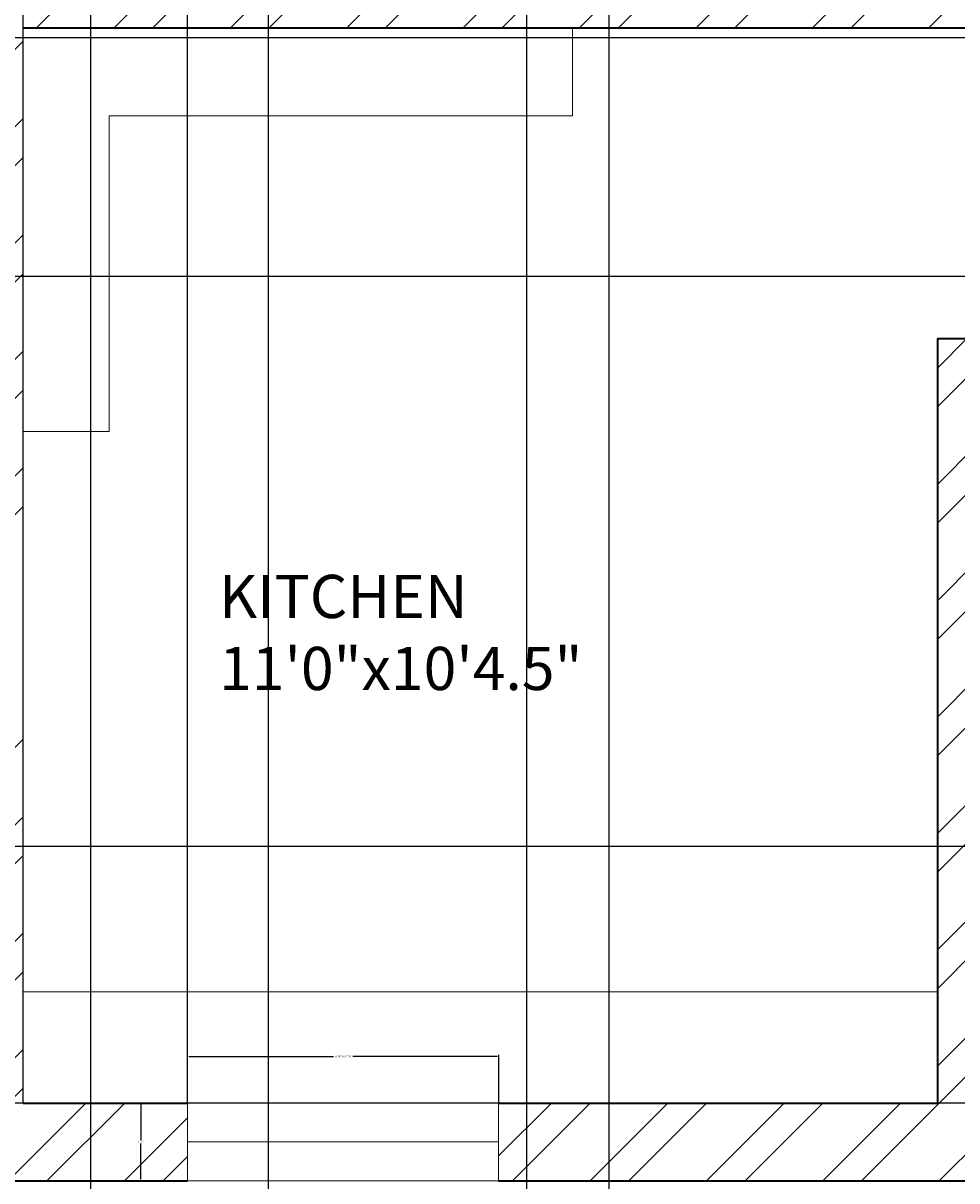
# Model space of a CAD drawing. Units: inches. Extents: x 1748 to 2382, y 1346 to 2284.
# Tile 3 of 26: x 1901 to 2009, y 1468 to 1602. Entities that reach past the tile are written whole.
import ezdxf

# ---------------------------------------------------------------- set-up
doc = ezdxf.new("R2010")
doc.units = ezdxf.units.IN
for name, color, linetype, lineweight in [('A-ANNO-DIMS', 2, 'Continuous', 18), ('A-AREA-IDEN', 7, 'Continuous', 18), ('A-FLOR-CASE', 32, 'Continuous', 18), ('A-GLAZ', 191, 'Continuous', 18), ('A-WALL', 7, 'Continuous', 35), ('A-WALL-PATT', 9, 'Continuous', 13)]:
    doc.layers.add(name, color=color, linetype=linetype, lineweight=lineweight)
doc.styles.get("Standard").update_dxf_attribs({"font": 'arial.ttf'})
doc.dimstyles.get("Standard").update_dxf_attribs({"dimtxt": 0.18, "dimasz": 0.18, "dimexe": 0.18, "dimexo": 0.0625, "dimgap": 0.09, "dimtad": 0, "dimtih": 1, "dimtoh": 1, "dimdec": 4, "dimzin": 0, "dimdsep": 46, "dimtxsty": 'Standard', "dimcen": 0.09, "dimadec": 0, "dimazin": 0, "dimtfac": 1, "dimtdec": 4, "dimtofl": 0, "dimtmove": 0, "dimatfit": 3, "dimfxl": 1, "dimtolj": 1, "dimtzin": 0, "dimarcsym": 0})

# ---------------------------------------------------------------- blocks, each defined once
blk = doc.blocks.new('WIN-36-DEEP')
for p, q in [((0, 9), (0, 0)), ((0, 9), (36, 9)), ((36, 4.5), (36, 9)), ((36, 9), (36, 0)), ((0, 0), (0, 4.5)), ((0, 4.5), (36, 4.5)), ((36, 0), (0, 0))]:
    blk.add_line(p, q)
blk = doc.blocks.new('*D28')
at = {"layer": 'A-ANNO-DIMS', "color": 0, "lineweight": -2, "transparency": 16777216}
for p, q in [((1919.68, 1476.91), (1919.68, 1482.43)), ((1955.68, 1476.91), (1955.68, 1482.43)), ((1919.86, 1482.25), (1936.56, 1482.25)), ((1955.5, 1482.25), (1938.8, 1482.25))]:
    blk.add_line(p, q, dxfattribs=at)
at = {"layer": 'A-ANNO-DIMS', "color": 0, "transparency": 16777216}
for points in [[(1919.86, 1482.28), (1919.86, 1482.22), (1919.68, 1482.25)], [(1955.5, 1482.28), (1955.5, 1482.22), (1955.68, 1482.25)]]:
    blk.add_solid(points, dxfattribs=at)
at = {"layer": 'Defpoints', "color": 0, "transparency": 16777216}
for p in [(1955.68, 1482.25), (1919.68, 1476.85), (1955.68, 1476.85)]:
    blk.add_point(p, dxfattribs=at)
at = {"layer": 'A-ANNO-DIMS', "color": 0, "transparency": 16777216, "insert": (1937.68, 1482.25), "char_height": 0.18, "attachment_point": 5}
blk.add_mtext('\\A1;WINDOW 36 TYP.', dxfattribs=at)
blk = doc.blocks.new('*D29')
at = {"layer": 'A-ANNO-DIMS', "color": 0, "lineweight": -2, "transparency": 16777216}
for p, q in [((1919.62, 1476.85), (1914.1, 1476.85)), ((1914.28, 1476.67), (1914.28, 1472.53)), ((1914.28, 1468.03), (1914.28, 1472.17)), ((1919.62, 1467.85), (1914.1, 1467.85))]:
    blk.add_line(p, q, dxfattribs=at)
at = {"layer": 'A-ANNO-DIMS', "color": 0, "transparency": 16777216}
for points in [[(1914.25, 1476.67), (1914.31, 1476.67), (1914.28, 1476.85)], [(1914.25, 1468.03), (1914.31, 1468.03), (1914.28, 1467.85)]]:
    blk.add_solid(points, dxfattribs=at)
at = {"layer": 'Defpoints', "color": 0, "transparency": 16777216}
for p in [(1914.28, 1476.85), (1919.68, 1476.85), (1919.68, 1467.85)]:
    blk.add_point(p, dxfattribs=at)
at = {"layer": 'A-ANNO-DIMS', "color": 0, "transparency": 16777216, "insert": (1914.28, 1472.35), "char_height": 0.18, "attachment_point": 5}
blk.add_mtext('\\A1;9 TYP.', dxfattribs=at)
blk = doc.blocks.new('*D50')
at = {"layer": 'A-ANNO-DIMS', "color": 0, "lineweight": -2, "transparency": 16777216}
for p, q in [((1869.96, 2223.79), (1869.96, 1360.47)), ((1908.44, 2223.79), (1908.44, 1360.47)), ((1870.14, 1360.65), (1888.81, 1360.65)), ((1908.26, 1360.65), (1889.6, 1360.65))]:
    blk.add_line(p, q, dxfattribs=at)
at = {"layer": 'A-ANNO-DIMS', "color": 0, "transparency": 16777216}
for points in [[(1870.14, 1360.68), (1870.14, 1360.62), (1869.96, 1360.65)], [(1908.26, 1360.68), (1908.26, 1360.62), (1908.44, 1360.65)]]:
    blk.add_solid(points, dxfattribs=at)
at = {"layer": 'Defpoints', "color": 0, "transparency": 16777216}
for p in [(1869.96, 2223.85), (1908.44, 2223.85), (1908.44, 1360.65)]:
    blk.add_point(p, dxfattribs=at)
at = {"layer": 'A-ANNO-DIMS', "color": 0, "transparency": 16777216, "insert": (1889.2, 1360.65), "char_height": 0.18, "attachment_point": 5}
blk.add_mtext('\\A1;38.48', dxfattribs=at)
blk = doc.blocks.new('*D51')
at = {"layer": 'A-ANNO-DIMS', "color": 0, "lineweight": -2, "transparency": 16777216}
for p, q in [((1968.44, 2223.79), (1968.44, 1360.47)), ((2040.07, 2223.79), (2040.07, 1360.47)), ((1968.62, 1360.65), (2003.86, 1360.65)), ((2039.89, 1360.65), (2004.65, 1360.65))]:
    blk.add_line(p, q, dxfattribs=at)
at = {"layer": 'A-ANNO-DIMS', "color": 0, "transparency": 16777216}
for points in [[(1968.62, 1360.68), (1968.62, 1360.62), (1968.44, 1360.65)], [(2039.89, 1360.68), (2039.89, 1360.62), (2040.07, 1360.65)]]:
    blk.add_solid(points, dxfattribs=at)
at = {"layer": 'Defpoints', "color": 0, "transparency": 16777216}
for p in [(1968.44, 2223.85), (2040.07, 2223.85), (2040.07, 1360.65)]:
    blk.add_point(p, dxfattribs=at)
at = {"layer": 'A-ANNO-DIMS', "color": 0, "transparency": 16777216, "insert": (2004.26, 1360.65), "char_height": 0.18, "attachment_point": 5}
blk.add_mtext('\\A1;71.62', dxfattribs=at)
blk = doc.blocks.new('*D54')
at = {"layer": 'A-ANNO-DIMS', "color": 0, "lineweight": -2, "transparency": 16777216}
for p, q in [((2288.4, 1506.57), (1779.88, 1506.57)), ((1780.06, 1506.39), (1780.06, 1491.89)), ((1780.06, 1477.03), (1780.06, 1491.53)), ((2288.4, 1476.85), (1779.88, 1476.85))]:
    blk.add_line(p, q, dxfattribs=at)
at = {"layer": 'A-ANNO-DIMS', "color": 0, "transparency": 16777216}
for points in [[(1780.03, 1506.39), (1780.09, 1506.39), (1780.06, 1506.57)], [(1780.03, 1477.03), (1780.09, 1477.03), (1780.06, 1476.85)]]:
    blk.add_solid(points, dxfattribs=at)
at = {"layer": 'Defpoints', "color": 0, "transparency": 16777216}
for p in [(1780.06, 1506.57), (2288.46, 1506.57), (2288.46, 1476.85)]:
    blk.add_point(p, dxfattribs=at)
at = {"layer": 'A-ANNO-DIMS', "color": 0, "transparency": 16777216, "insert": (1780.06, 1491.71), "char_height": 0.18, "attachment_point": 5}
blk.add_mtext('\\A1;29.716', dxfattribs=at)
blk = doc.blocks.new('*D64')
at = {"layer": 'A-ANNO-DIMS', "color": 0, "lineweight": -2, "transparency": 16777216}
for p, q in [((1900.64, 1476.91), (1900.64, 2274.93)), ((1900.82, 2274.75), (1909.7, 2274.75)), ((1919.5, 2274.75), (1910.62, 2274.75)), ((1919.68, 1476.91), (1919.68, 2274.93))]:
    blk.add_line(p, q, dxfattribs=at)
at = {"layer": 'A-ANNO-DIMS', "color": 0, "transparency": 16777216}
for points in [[(1900.82, 2274.78), (1900.82, 2274.72), (1900.64, 2274.75)], [(1919.5, 2274.78), (1919.5, 2274.72), (1919.68, 2274.75)]]:
    blk.add_solid(points, dxfattribs=at)
at = {"layer": 'Defpoints', "color": 0, "transparency": 16777216}
for p in [(1919.68, 2274.75), (1900.64, 1476.85), (1919.68, 1476.85)]:
    blk.add_point(p, dxfattribs=at)
at = {"layer": 'A-ANNO-DIMS', "color": 0, "transparency": 16777216, "insert": (1910.16, 2274.75), "char_height": 0.18, "attachment_point": 5}
blk.add_mtext('\\A1;19.035', dxfattribs=at)
blk = doc.blocks.new('*D79')
at = {"layer": 'A-ANNO-DIMS', "color": 0, "lineweight": -2, "transparency": 16777216}
for p, q in [((1929, 1854.79), (1929, 1360.47)), ((1958.9, 1854.79), (1958.9, 1360.47)), ((1929.18, 1360.65), (1943.62, 1360.65)), ((1958.72, 1360.65), (1944.27, 1360.65))]:
    blk.add_line(p, q, dxfattribs=at)
at = {"layer": 'A-ANNO-DIMS', "color": 0, "transparency": 16777216}
for points in [[(1929.18, 1360.68), (1929.18, 1360.62), (1929, 1360.65)], [(1958.72, 1360.68), (1958.72, 1360.62), (1958.9, 1360.65)]]:
    blk.add_solid(points, dxfattribs=at)
at = {"layer": 'Defpoints', "color": 0, "transparency": 16777216}
for p in [(1929, 1854.85), (1958.9, 1854.85), (1958.9, 1360.65)]:
    blk.add_point(p, dxfattribs=at)
at = {"layer": 'A-ANNO-DIMS', "color": 0, "transparency": 16777216, "insert": (1943.95, 1360.65), "char_height": 0.18, "attachment_point": 5}
blk.add_mtext('\\A1;29.9', dxfattribs=at)
blk = doc.blocks.new('*D80')
at = {"layer": 'A-ANNO-DIMS', "color": 0, "lineweight": -2, "transparency": 16777216}
for p, q in [((2058.9, 1600.19), (1779.88, 1600.19)), ((1780.06, 1600.01), (1780.06, 1586.55)), ((1780.06, 1572.73), (1780.06, 1586.19)), ((2058.9, 1572.55), (1779.88, 1572.55))]:
    blk.add_line(p, q, dxfattribs=at)
at = {"layer": 'A-ANNO-DIMS', "color": 0, "transparency": 16777216}
for points in [[(1780.03, 1600.01), (1780.09, 1600.01), (1780.06, 1600.19)], [(1780.03, 1572.73), (1780.09, 1572.73), (1780.06, 1572.55)]]:
    blk.add_solid(points, dxfattribs=at)
at = {"layer": 'Defpoints', "color": 0, "transparency": 16777216}
for p in [(1780.06, 1600.19), (2058.96, 1600.19), (2058.96, 1572.55)]:
    blk.add_point(p, dxfattribs=at)
at = {"layer": 'A-ANNO-DIMS', "color": 0, "transparency": 16777216, "insert": (1780.06, 1586.37), "char_height": 0.18, "attachment_point": 5}
blk.add_mtext('\\A1;27.637', dxfattribs=at)

msp = doc.modelspace()

# ---------------------------------------------------------------- hatches: boundary and pattern name
at = {"layer": 'A-WALL-PATT'}
h = msp.add_hatch(dxfattribs=at)
h.set_pattern_fill('ANSI32', color=256)
h.paths.add_polyline_path([(1908.4445, 2232.8497), (1821.9607, 2232.8497), (1821.9607, 2223.8497), (1865.4607, 2223.8497), (1865.4607, 2209.9185), (1869.9607, 2209.9185), (1869.9607, 2223.8497), (1908.4445, 2223.8497), (1908.4445, 2228.3497)])
h.paths.add_polyline_path([(2040.0683, 2232.8497), (1968.4445, 2232.8497), (1968.4445, 2223.8497), (2025.9607, 2223.8497), (2025.9607, 2130.3497), (2032.1341, 2130.3497), (2032.1341, 2132.5997), (2032.1341, 2134.8497), (2030.4607, 2134.8497), (2030.4607, 2223.8497), (2040.0683, 2223.8497)])
h.paths.add_polyline_path([(2091.3969, 2232.8497), (2064.0683, 2232.8497), (2064.0683, 2223.8497), (2078.4607, 2223.8497), (2078.4607, 2134.8497), (2051.1563, 2134.8497), (2051.1563, 2130.3497), (2078.4607, 2130.3497), (2078.4607, 2128.6813), (2082.9607, 2128.6813), (2082.9607, 2130.3497), (2086.1879, 2130.3497), (2086.1879, 2132.5997), (2086.1879, 2134.8497), (2082.9607, 2134.8497), (2082.9607, 2223.8497), (2091.3969, 2223.8497), (2091.3969, 2228.3497)])
h.paths.add_polyline_path([(2167.0164, 2232.8497), (2115.3969, 2232.8497), (2115.3969, 2223.8497), (2130.9607, 2223.8497), (2130.9607, 2134.8497), (2106.9607, 2134.8497), (2106.9607, 2130.3497), (2135.4607, 2130.3497), (2135.4607, 2223.8497), (2167.0164, 2223.8497), (2167.0164, 2228.3497)])
h.paths.add_polyline_path([(1869.9607, 2149.9185), (1865.4607, 2149.9185), (1865.4607, 2127.8942), (1869.9607, 2127.8942)])
h.paths.add_polyline_path([(2082.9607, 2104.4871), (2080.7107, 2104.4871), (2078.4607, 2104.4871), (2078.4607, 2103.8497), (1869.9607, 2103.8497), (1869.9607, 2108.6062), (1867.7107, 2108.6062), (1865.4607, 2108.6062), (1865.4607, 2103.8497), (1821.9607, 2103.8497), (1821.9607, 2099.3497), (1865.4607, 2099.3497), (1865.4607, 2094.7509), (1869.9607, 2094.7509), (1869.9607, 2099.3497), (2025.9607, 2099.3497), (2025.9607, 2096.4326), (2030.4607, 2096.4326), (2030.4607, 2099.3497), (2082.9607, 2099.3497)])
h.paths.add_polyline_path([(1928.9457, 1401.1212), (2176.8693, 1401.1212), (2176.8693, 1438.214), (1928.9457, 1438.214)], flags=9)
h.paths.add_polyline_path([(2122.2668, 2048.1927), (2177.9387, 2048.1927), (2177.9387, 2066.85), (2122.2668, 2066.85)], flags=9)
h.paths.add_polyline_path([(2272.688, 2153.8197), (2272.688, 2216.746), (2262.3845, 2216.746), (2262.3845, 2153.8197)], flags=9)
h.paths.add_polyline_path([(2157.2928, 2166.5593), (2196.3822, 2166.5593), (2196.3822, 2185.2167), (2157.2928, 2185.2167)], flags=9)
h.paths.add_polyline_path([(2089.3407, 2162.0698), (2124.3987, 2162.0698), (2124.3987, 2180.7272), (2089.3407, 2180.7272)], flags=9)
h.paths.add_polyline_path([(2037.4521, 2160.0913), (2072.5101, 2160.0913), (2072.5101, 2178.7486), (2037.4521, 2178.7486)], flags=9)
h.paths.add_polyline_path([(1884.7894, 2104.1554), (1923.6297, 2104.1554), (1923.6297, 2122.8127), (1884.7894, 2122.8127)], flags=9)
h.paths.add_polyline_path([(1851.2832, 2142.9749), (1851.2832, 2199.3051), (1840.9796, 2199.3051), (1840.9796, 2142.9749)], flags=9)
h.paths.add_polyline_path([(1844.8763, 2017.2834), (1844.8763, 2073.6136), (1834.5728, 2073.6136), (1834.5728, 2017.2834)], flags=9)
h.paths.add_polyline_path([(1897.1577, 2073.1279), (1935.9981, 2073.1279), (1935.9981, 2091.7853), (1897.1577, 2091.7853)], flags=9)
h.paths.add_polyline_path([(1952.3395, 1802.4231), (2008.0114, 1802.4231), (2008.0114, 1821.0805), (1952.3395, 1821.0805)], flags=9)
h.paths.add_polyline_path([(1978.8184, 1857.6841), (2017.7338, 1857.6841), (2017.7338, 1876.3415), (1978.8184, 1876.3415)], flags=9)
h.paths.add_polyline_path([(1979.6513, 1925.9516), (2008.8089, 1925.9516), (2008.8089, 1944.6089), (1979.6513, 1944.6089)], flags=9)
h.paths.add_polyline_path([(1838.5553, 1860.3527), (1877.3957, 1860.3527), (1877.3957, 1879.01), (1838.5553, 1879.01)], flags=9)
h.paths.add_polyline_path([(1883.9018, 1787.3013), (1883.9018, 1843.6315), (1873.5983, 1843.6315), (1873.5983, 1787.3013)], flags=9)
h.paths.add_polyline_path([(1873.7079, 1509.1938), (1873.7079, 1583.7709), (1863.4044, 1583.7709), (1863.4044, 1509.1938)], flags=9)
h.paths.add_polyline_path([(1916.2259, 1603.3681), (1955.0663, 1603.3681), (1955.0663, 1622.0254), (1916.2259, 1622.0254)], flags=9)
h.paths.add_polyline_path([(1876.3013, 1636.757), (1876.3013, 1693.0871), (1865.9978, 1693.0871), (1865.9978, 1636.757)], flags=9)
h.paths.add_polyline_path([(1921.3138, 1521.8316), (1964.0662, 1521.8316), (1964.0662, 1540.489), (1921.3138, 1540.489)], flags=9)
h.paths.add_polyline_path([(2017.5657, 1497.5078), (2046.7983, 1497.5078), (2046.7983, 1516.1651), (2017.5657, 1516.1651)], flags=9)
h.paths.add_polyline_path([(2066.8661, 1499.3902), (2096.0988, 1499.3902), (2096.0988, 1518.0475), (2066.8661, 1518.0475)], flags=9)
h.paths.add_polyline_path([(2155.4835, 1571.6596), (2198.2358, 1571.6596), (2198.2358, 1590.3169), (2155.4835, 1590.3169)], flags=9)
h.paths.add_polyline_path([(2094.9136, 1664.6812), (2150.5855, 1664.6812), (2150.5855, 1683.3386), (2094.9136, 1683.3386)], flags=9)
h.paths.add_polyline_path([(2257.6902, 1863.1628), (2269.8935, 1863.1628), (2269.8935, 1873.4664), (2257.6902, 1873.4664)], flags=9)
h.paths.add_polyline_path([(2164.0748, 1880.3089), (2189.8694, 1880.3089), (2189.8694, 1890.6124), (2164.0748, 1890.6124)], flags=9)
h.paths.add_polyline_path([(2239.4394, 1931.0585), (2268.8187, 1931.0585), (2268.8187, 1949.7159), (2239.4394, 1949.7159)], flags=9)
h = msp.add_hatch(dxfattribs=at)
h.set_pattern_fill('ANSI32', color=256)
h.paths.add_polyline_path([(2297.4607, 2232.8497), (2203.0164, 2232.8497), (2203.0164, 2223.8497), (2244.9607, 2223.8497), (2244.9607, 2127.8554), (2249.4607, 2127.8554), (2249.4607, 2223.8497), (2297.4607, 2223.8497)])
h.paths.add_polyline_path([(2297.4607, 2103.8497), (2249.4607, 2103.8497), (2249.4607, 2106.7497), (2247.2107, 2106.7497), (2244.9607, 2106.7497), (2244.9607, 2103.8497), (2130.9607, 2103.8497), (2130.9607, 2099.3497), (2288.4607, 2099.3497), (2288.4607, 2077.2008), (2297.4607, 2077.2008)])
h.paths.add_polyline_path([(1928.9457, 1401.1212), (2176.8693, 1401.1212), (2176.8693, 1438.214), (1928.9457, 1438.214)], flags=9)
h.paths.add_polyline_path([(2122.2668, 2048.1927), (2177.9387, 2048.1927), (2177.9387, 2066.85), (2122.2668, 2066.85)], flags=9)
h.paths.add_polyline_path([(2272.688, 2153.8197), (2272.688, 2216.746), (2262.3845, 2216.746), (2262.3845, 2153.8197)], flags=25)
h.paths.add_polyline_path([(2157.2928, 2166.5593), (2196.3822, 2166.5593), (2196.3822, 2185.2167), (2157.2928, 2185.2167)], flags=9)
h.paths.add_polyline_path([(2089.3407, 2162.0698), (2124.3987, 2162.0698), (2124.3987, 2180.7272), (2089.3407, 2180.7272)], flags=9)
h.paths.add_polyline_path([(2037.4521, 2160.0913), (2072.5101, 2160.0913), (2072.5101, 2178.7486), (2037.4521, 2178.7486)], flags=9)
h.paths.add_polyline_path([(1884.7894, 2104.1554), (1923.6297, 2104.1554), (1923.6297, 2122.8127), (1884.7894, 2122.8127)], flags=9)
h.paths.add_polyline_path([(1851.2832, 2142.9749), (1851.2832, 2199.3051), (1840.9796, 2199.3051), (1840.9796, 2142.9749)], flags=9)
h.paths.add_polyline_path([(1844.8763, 2017.2834), (1844.8763, 2073.6136), (1834.5728, 2073.6136), (1834.5728, 2017.2834)], flags=9)
h.paths.add_polyline_path([(1897.1577, 2073.1279), (1935.9981, 2073.1279), (1935.9981, 2091.7853), (1897.1577, 2091.7853)], flags=9)
h.paths.add_polyline_path([(1952.3395, 1802.4231), (2008.0114, 1802.4231), (2008.0114, 1821.0805), (1952.3395, 1821.0805)], flags=9)
h.paths.add_polyline_path([(1978.8184, 1857.6841), (2017.7338, 1857.6841), (2017.7338, 1876.3415), (1978.8184, 1876.3415)], flags=9)
h.paths.add_polyline_path([(1979.6513, 1925.9516), (2008.8089, 1925.9516), (2008.8089, 1944.6089), (1979.6513, 1944.6089)], flags=9)
h.paths.add_polyline_path([(1838.5553, 1860.3527), (1877.3957, 1860.3527), (1877.3957, 1879.01), (1838.5553, 1879.01)], flags=9)
h.paths.add_polyline_path([(1883.9018, 1787.3013), (1883.9018, 1843.6315), (1873.5983, 1843.6315), (1873.5983, 1787.3013)], flags=9)
h.paths.add_polyline_path([(1873.7079, 1509.1938), (1873.7079, 1583.7709), (1863.4044, 1583.7709), (1863.4044, 1509.1938)], flags=9)
h.paths.add_polyline_path([(1916.2259, 1603.3681), (1955.0663, 1603.3681), (1955.0663, 1622.0254), (1916.2259, 1622.0254)], flags=9)
h.paths.add_polyline_path([(1876.3013, 1636.757), (1876.3013, 1693.0871), (1865.9978, 1693.0871), (1865.9978, 1636.757)], flags=9)
h.paths.add_polyline_path([(1921.3138, 1521.8316), (1964.0662, 1521.8316), (1964.0662, 1540.489), (1921.3138, 1540.489)], flags=9)
h.paths.add_polyline_path([(2017.5657, 1497.5078), (2046.7983, 1497.5078), (2046.7983, 1516.1651), (2017.5657, 1516.1651)], flags=9)
h.paths.add_polyline_path([(2066.8661, 1499.3902), (2096.0988, 1499.3902), (2096.0988, 1518.0475), (2066.8661, 1518.0475)], flags=9)
h.paths.add_polyline_path([(2155.4835, 1571.6596), (2198.2358, 1571.6596), (2198.2358, 1590.3169), (2155.4835, 1590.3169)], flags=9)
h.paths.add_polyline_path([(2094.9136, 1664.6812), (2150.5855, 1664.6812), (2150.5855, 1683.3386), (2094.9136, 1683.3386)], flags=9)
h.paths.add_polyline_path([(2257.6902, 1863.1628), (2269.8935, 1863.1628), (2269.8935, 1873.4664), (2257.6902, 1873.4664)], flags=9)
h.paths.add_polyline_path([(2164.0748, 1880.3089), (2189.8694, 1880.3089), (2189.8694, 1890.6124), (2164.0748, 1890.6124)], flags=9)
h.paths.add_polyline_path([(2239.4394, 1931.0585), (2268.8187, 1931.0585), (2268.8187, 1949.7159), (2239.4394, 1949.7159)], flags=9)
h = msp.add_hatch(dxfattribs=at)
h.set_pattern_fill('ANSI32', color=256)
h.paths.add_polyline_path([(1919.6777, 1476.8497), (1900.6426, 1476.8497), (1900.6426, 1522.0826), (1898.3926, 1522.0826), (1896.1426, 1522.0826), (1896.1426, 1476.8497), (1857.1426, 1476.8497), (1857.1426, 1467.8497), (1896.1426, 1467.8497), (1919.6777, 1467.8497), (1919.6777, 1472.3497)])
h.paths.add_polyline_path([(2018.7873, 1472.3497), (2018.7873, 1476.8497), (2010.9607, 1476.8497), (2010.9607, 1560.8497), (2034.9607, 1560.8497), (2034.9607, 1565.3497), (2006.4607, 1565.3497), (2006.4607, 1476.8497), (1955.6777, 1476.8497), (1955.6777, 1467.8497), (2018.7873, 1467.8497)])
h.paths.add_polyline_path([(2152.3354, 1472.3497), (2152.3354, 1476.8497), (2115.9607, 1476.8497), (2115.9607, 1565.3497), (2109.2204, 1565.3497), (2109.2204, 1563.0997), (2109.2204, 1560.8497), (2111.4607, 1560.8497), (2111.4607, 1476.8497), (2095.3617, 1476.8497), (2095.3617, 1467.8497), (2152.3354, 1467.8497)])
h.paths.add_polyline_path([(2071.3617, 1476.8497), (2063.4607, 1476.8497), (2063.4607, 1560.8497), (2090.1865, 1560.8497), (2090.1865, 1565.3497), (2063.4607, 1565.3497), (2063.4607, 1572.5485), (2061.2107, 1572.5485), (2058.9607, 1572.5485), (2058.9607, 1565.3497), (2055.6281, 1565.3497), (2055.6281, 1560.8497), (2058.9607, 1560.8497), (2058.9607, 1476.8497), (2042.7873, 1476.8497), (2042.7873, 1467.8497), (2071.3617, 1467.8497), (2071.3617, 1472.3497)])
h.paths.add_polyline_path([(2297.4607, 1506.5652), (2288.4607, 1506.5652), (2288.4607, 1476.8497), (2212.3354, 1476.8497), (2212.3354, 1467.8497), (2297.4607, 1467.8497)])
h.paths.add_polyline_path([(2297.4607, 1645.3038), (2288.4607, 1645.3038), (2288.4607, 1605.8497), (2058.9607, 1605.8497), (2058.9607, 1600.1857), (2061.2107, 1600.1857), (2063.4607, 1600.1857), (2063.4607, 1601.3497), (2288.4607, 1601.3497), (2288.4607, 1566.5652), (2297.4607, 1566.5652)])
h.paths.add_polyline_path([(2010.9607, 1609.0561), (2008.7107, 1609.0561), (2006.4607, 1609.0561), (2006.4607, 1605.8497), (1900.6426, 1605.8497), (1900.6426, 1609.7171), (1898.3926, 1609.7171), (1896.1426, 1609.7171), (1896.1426, 1605.8497), (1857.1426, 1605.8497), (1857.1426, 1601.3497), (1896.1426, 1601.3497), (1896.1426, 1542.5447), (1900.6426, 1542.5447), (1900.6426, 1601.3497), (2010.9607, 1601.3497)])
h.paths.add_polyline_path([(1928.9457, 1401.1212), (2176.8693, 1401.1212), (2176.8693, 1438.214), (1928.9457, 1438.214)], flags=9)
h.paths.add_polyline_path([(2122.2668, 2048.1927), (2177.9387, 2048.1927), (2177.9387, 2066.85), (2122.2668, 2066.85)], flags=9)
h.paths.add_polyline_path([(2272.688, 2153.8197), (2272.688, 2216.746), (2262.3845, 2216.746), (2262.3845, 2153.8197)], flags=9)
h.paths.add_polyline_path([(2157.2928, 2166.5593), (2196.3822, 2166.5593), (2196.3822, 2185.2167), (2157.2928, 2185.2167)], flags=9)
h.paths.add_polyline_path([(2089.3407, 2162.0698), (2124.3987, 2162.0698), (2124.3987, 2180.7272), (2089.3407, 2180.7272)], flags=9)
h.paths.add_polyline_path([(2037.4521, 2160.0913), (2072.5101, 2160.0913), (2072.5101, 2178.7486), (2037.4521, 2178.7486)], flags=9)
h.paths.add_polyline_path([(1884.7894, 2104.1554), (1923.6297, 2104.1554), (1923.6297, 2122.8127), (1884.7894, 2122.8127)], flags=9)
h.paths.add_polyline_path([(1851.2832, 2142.9749), (1851.2832, 2199.3051), (1840.9796, 2199.3051), (1840.9796, 2142.9749)], flags=9)
h.paths.add_polyline_path([(1844.8763, 2017.2834), (1844.8763, 2073.6136), (1834.5728, 2073.6136), (1834.5728, 2017.2834)], flags=9)
h.paths.add_polyline_path([(1897.1577, 2073.1279), (1935.9981, 2073.1279), (1935.9981, 2091.7853), (1897.1577, 2091.7853)], flags=9)
h.paths.add_polyline_path([(1952.3395, 1802.4231), (2008.0114, 1802.4231), (2008.0114, 1821.0805), (1952.3395, 1821.0805)], flags=9)
h.paths.add_polyline_path([(1978.8184, 1857.6841), (2017.7338, 1857.6841), (2017.7338, 1876.3415), (1978.8184, 1876.3415)], flags=9)
h.paths.add_polyline_path([(1979.6513, 1925.9516), (2008.8089, 1925.9516), (2008.8089, 1944.6089), (1979.6513, 1944.6089)], flags=9)
h.paths.add_polyline_path([(1838.5553, 1860.3527), (1877.3957, 1860.3527), (1877.3957, 1879.01), (1838.5553, 1879.01)], flags=9)
h.paths.add_polyline_path([(1883.9018, 1787.3013), (1883.9018, 1843.6315), (1873.5983, 1843.6315), (1873.5983, 1787.3013)], flags=9)
h.paths.add_polyline_path([(1873.7079, 1509.1938), (1873.7079, 1583.7709), (1863.4044, 1583.7709), (1863.4044, 1509.1938)], flags=9)
h.paths.add_polyline_path([(1916.2259, 1603.3681), (1955.0663, 1603.3681), (1955.0663, 1622.0254), (1916.2259, 1622.0254)], flags=9)
h.paths.add_polyline_path([(1876.3013, 1636.757), (1876.3013, 1693.0871), (1865.9978, 1693.0871), (1865.9978, 1636.757)], flags=9)
h.paths.add_polyline_path([(1921.3138, 1521.8316), (1964.0662, 1521.8316), (1964.0662, 1540.489), (1921.3138, 1540.489)], flags=9)
h.paths.add_polyline_path([(2017.5657, 1497.5078), (2046.7983, 1497.5078), (2046.7983, 1516.1651), (2017.5657, 1516.1651)], flags=9)
h.paths.add_polyline_path([(2066.8661, 1499.3902), (2096.0988, 1499.3902), (2096.0988, 1518.0475), (2066.8661, 1518.0475)], flags=9)
h.paths.add_polyline_path([(2155.4835, 1571.6596), (2198.2358, 1571.6596), (2198.2358, 1590.3169), (2155.4835, 1590.3169)], flags=25)
h.paths.add_polyline_path([(2094.9136, 1664.6812), (2150.5855, 1664.6812), (2150.5855, 1683.3386), (2094.9136, 1683.3386)], flags=9)
h.paths.add_polyline_path([(2257.6902, 1863.1628), (2269.8935, 1863.1628), (2269.8935, 1873.4664), (2257.6902, 1873.4664)], flags=9)
h.paths.add_polyline_path([(2164.0748, 1880.3089), (2189.8694, 1880.3089), (2189.8694, 1890.6124), (2164.0748, 1890.6124)], flags=9)
h.paths.add_polyline_path([(2239.4394, 1931.0585), (2268.8187, 1931.0585), (2268.8187, 1949.7159), (2239.4394, 1949.7159)], flags=9)

# ---------------------------------------------------------------- linework, layer by layer
at = {"layer": 'A-FLOR-CASE'}
for p, q in [((1964.2445, 1593.352), (1964.2445, 1601.3497)), ((1964.2445, 1591.1355), (1964.2445, 1593.352)), ((1910.6107, 1554.5909), (1910.6107, 1591.1355)), ((1910.6107, 1591.1355), (1964.2445, 1591.1355)), ((1900.6426, 1554.5909), (1908.5437, 1554.5909)), ((1908.5437, 1554.5909), (1910.6107, 1554.5909)), ((1900.6426, 1489.7224), (2006.4607, 1489.7224))]:
    msp.add_line(p, q, dxfattribs=at)
at = {"layer": 'A-WALL'}
for p, q in [((1900.6426, 1601.3497), (2010.9607, 1601.3497)), ((2006.4607, 1565.3497), (2006.4607, 1476.8497)), ((2006.4607, 1565.3497), (2034.9607, 1565.3497)), ((1900.6426, 1476.8497), (1919.6777, 1476.8497)), ((1955.6777, 1476.8497), (2006.4607, 1476.8497)), ((1896.1426, 1467.8497), (1919.6777, 1467.8497)), ((1955.6777, 1467.8497), (2018.7873, 1467.8497))]:
    msp.add_line(p, q, dxfattribs=at)

# ---------------------------------------------------------------- block references
at = {"layer": 'A-GLAZ'}
msp.add_blockref('WIN-36-DEEP', (1919.678, 1467.85), dxfattribs=at)

# ---------------------------------------------------------------- texts
at = {"layer": 'A-AREA-IDEN', "insert": (1923.3244, 1538.0009), "char_height": 5, "attachment_point": 1}
msp.add_mtext_dynamic_manual_height_columns('KITCHEN\\P11\'0"x10\'4.5"', width=160.639926, gutter_width=12.5, heights=[0], dxfattribs=at)

# ---------------------------------------------------------------- dimensions: what is measured, and where the dimension line sits
at = {"layer": 'A-ANNO-DIMS'}
for base, p1, p2, override, picture, middle in [((1919.6777, 2274.7497), (1900.6426, 1476.8497), (1919.6777, 1476.8497), {"dimdec": 3, "dimlfac": 1, "dimrnd": 0, "dimzin": 0, "dimdsep": 46, "dimlunit": 2}, '*D64', (1910.1602, 2274.7497)), ((1908.4445, 1360.6451), (1869.9607, 2223.8497), (1908.4445, 2223.8497), {"dimdec": 2, "dimlfac": 1, "dimrnd": 0, "dimzin": 0, "dimdsep": 46, "dimlunit": 2}, '*D50', (1889.2026, 1360.6451)), ((2040.0683, 1360.6451), (1968.4445, 2223.8497), (2040.0683, 2223.8497), {"dimdec": 2, "dimlfac": 1, "dimrnd": 0, "dimzin": 0, "dimdsep": 46, "dimlunit": 2}, '*D51', (2004.2564, 1360.6451)), ((1958.8973, 1360.6451), (1928.9996, 1854.8497), (1958.8973, 1854.8497), {"dimdec": 1, "dimlfac": 1, "dimrnd": 0, "dimzin": 0, "dimdsep": 46, "dimlunit": 2}, '*D79', (1943.9485, 1360.6451))]:
    dim = msp.add_linear_dim(base=base, p1=p1, p2=p2, dimstyle='Standard', override=override, dxfattribs=at)
    dim.commit()
    dim.dimension.update_dxf_attribs({"geometry": picture, "text_midpoint": middle})
for base, p1, p2, picture, middle in [((1780.0607, 1600.1857), (2058.9607, 1572.5485), (2058.9607, 1600.1857), '*D80', (1780.0607, 1586.3671)), ((1780.06066, 1506.56516), (2288.46066, 1476.84965), (2288.46066, 1506.56516), '*D54', (1780.06066, 1491.7074))]:
    dim = msp.add_linear_dim(base=base, p1=p1, p2=p2, angle=90, dimstyle='Standard', override={"dimdec": 3, "dimlfac": 1, "dimrnd": 0, "dimzin": 0, "dimdsep": 46, "dimlunit": 2}, dxfattribs=at)
    dim.commit()
    dim.dimension.update_dxf_attribs({"geometry": picture, "text_midpoint": middle})
dim = msp.add_linear_dim(base=(1955.6777, 1482.2497), p1=(1919.6777, 1476.8497), p2=(1955.6777, 1476.8497), text='WINDOW <> TYP.', dimstyle='Standard', override={"dimdec": 0, "dimlfac": 1, "dimrnd": 0, "dimzin": 0, "dimdsep": 46, "dimlunit": 2}, dxfattribs=at)
dim.commit()
dim.dimension.update_dxf_attribs({"geometry": '*D28', "text_midpoint": (1937.6777, 1482.2497)})
dim = msp.add_linear_dim(base=(1914.2777, 1476.8497), p1=(1919.6777, 1467.8497), p2=(1919.6777, 1476.8497), angle=90, text='<> TYP.', dimstyle='Standard', override={"dimdec": 0, "dimlfac": 1, "dimrnd": 0, "dimzin": 0, "dimdsep": 46, "dimlunit": 2}, dxfattribs=at)
dim.commit()
dim.dimension.update_dxf_attribs({"geometry": '*D29', "text_midpoint": (1914.2777, 1472.3497)})

doc.saveas('drawing.dxf')
